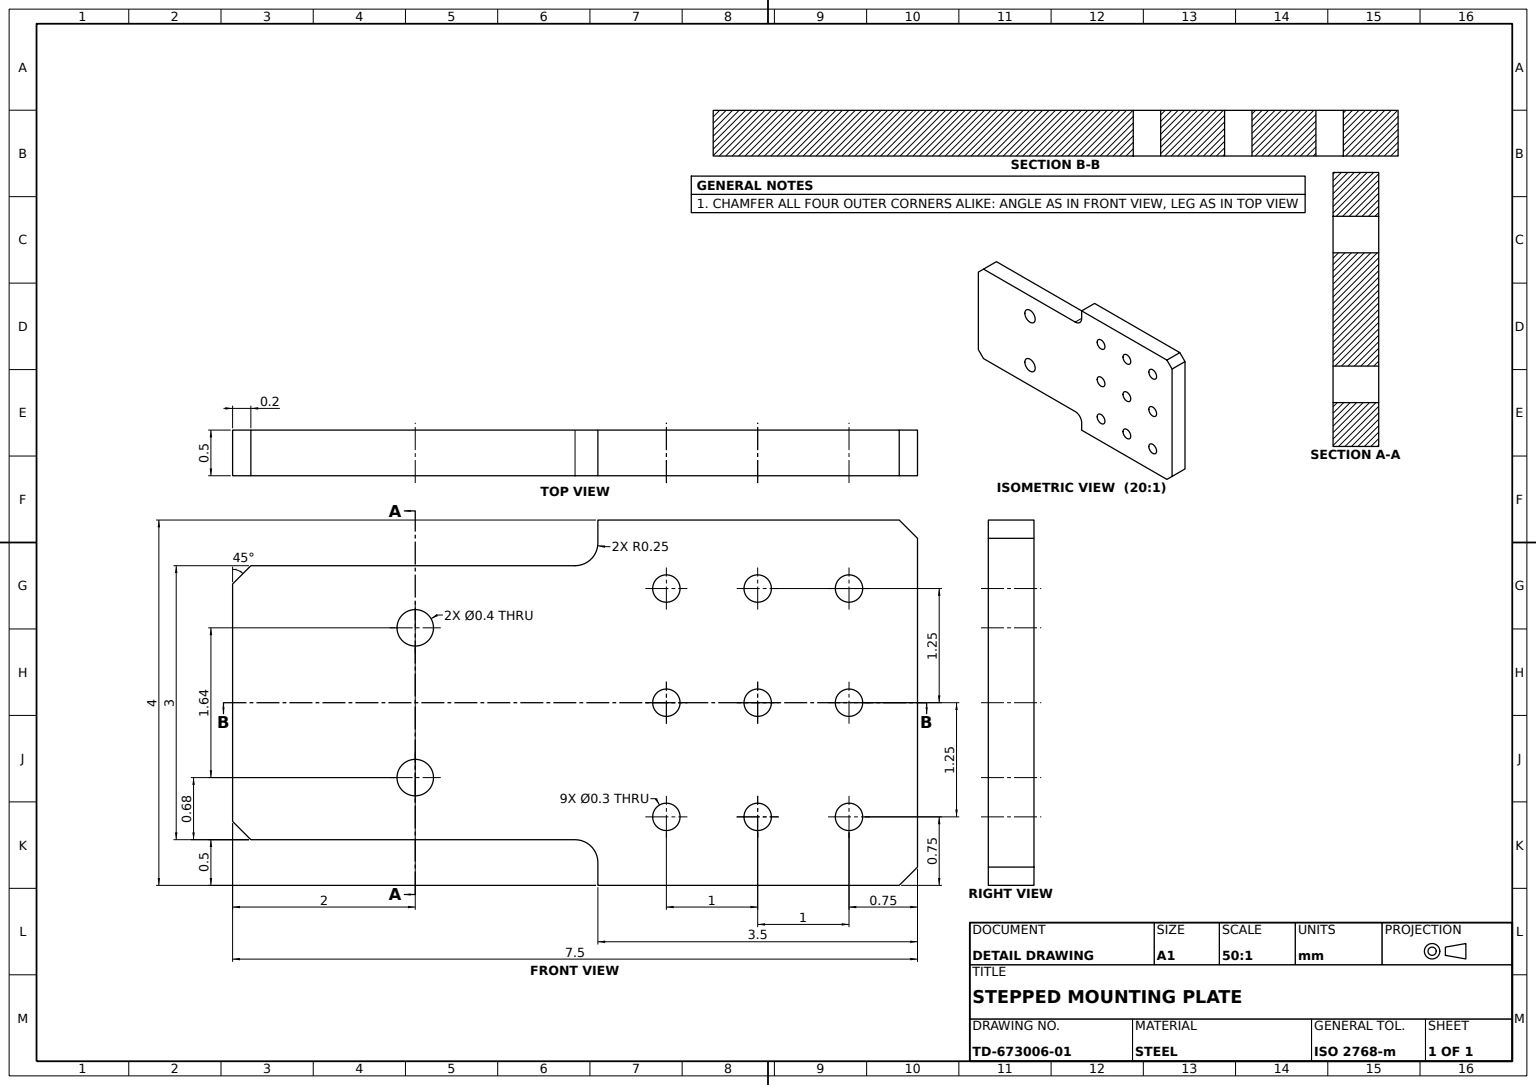
SolidWorks part; units mm, degrees
material "Plain Carbon Steel"
ref_plane "Front Plane" through (0, 0, 0) normal (0, 0, 1) x (1, 0, 0)
ref_plane "Top Plane" through (0, 0, 0) normal (0, 1, 0) x (1, 0, 0)
ref_plane "Right Plane" through (0, 0, 0) normal (1, 0, 0) x (0, 0, -1)
sketch "Stepped Tab Profile Sketch" plane through (0, 0, 0) normal (0, 0, 1) x (1, 0, 0)
  line L0 (0, 0) -> (7.5, 0)
  line L1 (7.5, 0) -> (7.5, 2)
  line L2 (7.5, 2) -> (4, 2)
  line L3 (7.5, 0) -> (7.5, -2)
  line L4 (7.5, -2) -> (4, -2)
  line L5 (0, 0) -> (0, 1.5)
  line L6 (0, 1.5) -> (3.75, 1.5)
  line L7 (4, 1.75) -> (4, 2)
  line L8 (0, 0) -> (0, -1.5)
  line L9 (0, -1.5) -> (3.75, -1.5)
  line L10 (4, -1.75) -> (4, -2)
  arc A0 (4, -1.75) -> (3.75, -1.5) centre (3.75, -1.75) ccw
  arc A1 (3.75, 1.5) -> (4, 1.75) centre (3.75, 1.75) ccw
  dimension "D3" = 3.5
  dimension "D8" = 0.25
  dimension "D1" = 7.5
  dimension "D2" = 2
  dimension "D4" = 2
  dimension "D5" = 3.5
  dimension "D6" = 1.5
  dimension "D7" = 1.5
extrude "Stepped Tab Plate 0.5mm" add sketch "Stepped Tab Profile Sketch" along normal blind 0.5 contours A1 L6 L5 L0 L1 L2 L7 | A0 L10 L4 L3 L0 L8 L9
chamfer "Corner Chamfer 0.2x45 A" distance 0.2 angle 45 2 edges at (0, 1.5, 0.25) (7.5, 2, 0.25)
chamfer "Corner Chamfer 0.2x45 B" distance 0.2 angle 45 2 edges at (7.5, -2, 0.25) (0, -1.5, 0.25)
sketch "Screw Holes Sketch" plane through (0, 0, 0.5) normal (0, 0, 1) x (1, 0, 0)
  line L0 (0, -1.3) -> (0, 1.3) construction
  line L1 (0.2, 1.5) -> (3.75, 1.5) construction
  line L2 (0.2, -1.5) -> (3.75, -1.5) construction
  circle A0 centre (2, 0.82) radius 0.2
  circle A1 centre (2, -0.82) radius 0.2
  dimension "D1" = 0.2
  dimension "D2" = 0.2
  dimension "D3" = 2
  dimension "D4" = 2
  dimension "D5" = 0.68
  dimension "D6" = 0.68
extrude "Screw Holes 2x" cut sketch "Screw Holes Sketch" against normal blind 1
sketch "Hole Grid Sketch" plane through (0, 0, 0.5) normal (0, 0, 1) x (1, 0, 0)
  line L0 (4, 1.75) -> (4, 2) construction
  line L2 (7.3, 2) -> (4, 2) construction
  line L3 (7.5, -1.8) -> (7.5, 1.8) construction
  circle A0 centre (4.75, 1.25) radius 0.15
  circle A1 centre (5.75, 1.25) radius 0.15
  circle A2 centre (6.75, 1.25) radius 0.15
  circle A3 centre (6.75, 0) radius 0.15
  circle A4 centre (6.75, -1.25) radius 0.15
  circle A5 centre (5.75, -1.25) radius 0.15
  circle A6 centre (4.75, -1.25) radius 0.15
  circle A7 centre (4.75, 0) radius 0.15
  circle A8 centre (5.75, 0) radius 0.15
  dimension "D1" = 0.15
  dimension "D2" = 0.15
  dimension "D3" = 0.15
  dimension "D4" = 0.15
  dimension "D5" = 0.15
  dimension "D6" = 0.15
  dimension "D7" = 0.15
  dimension "D8" = 0.15
  dimension "D9" = 0.15
  dimension "D10" = 0.75
  dimension "D11" = 0.75
  dimension "D12" = 0.75
  dimension "D13" = 0.75
  dimension "D14" = 0.75
  dimension "D15" = 1
  dimension "D16" = 0.75
  dimension "D17" = 1.25
  dimension "D18" = 1.25
  dimension "D19" = 1.25
  dimension "D20" = 1.25
  dimension "D21" = 1.25
  dimension "D22" = 1
  dimension "D23" = 1
  dimension "D24" = 0.75
  dimension "D25" = 1.25
  dimension "D26" = 1
  dimension "D27" = 1
extrude "Hole Grid 3x3" cut sketch "Hole Grid Sketch" against normal blind 1
